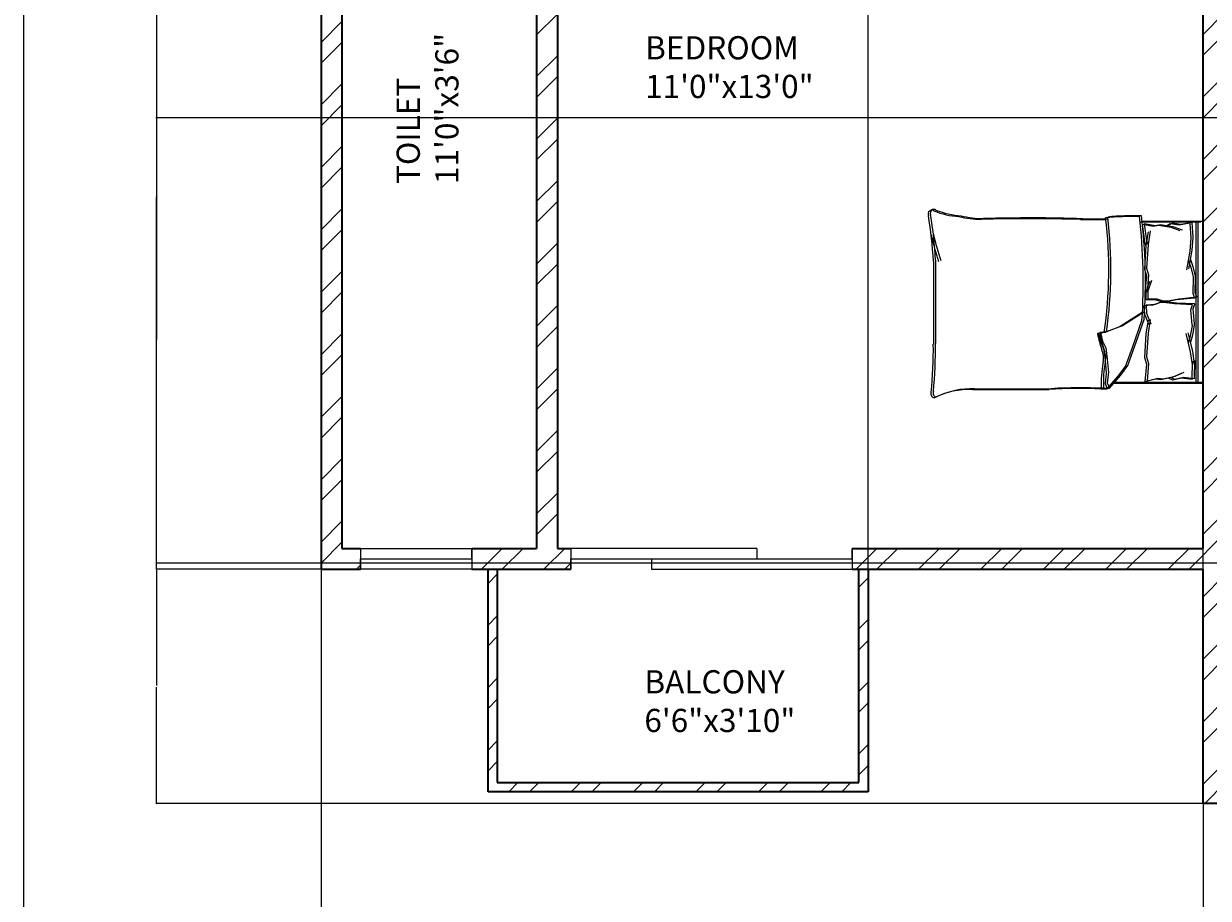
# Model space of a CAD drawing. Units: inches. Extents: x 2064 to 2782, y 1196 to 2299.
# Tile 2 of 11: x 2064 to 2320, y 1620 to 1809. Entities that reach past the tile are written whole.
import ezdxf

# ---------------------------------------------------------------- set-up
doc = ezdxf.new("R2010")
doc.units = ezdxf.units.IN
for name, color, linetype, lineweight in [('A-ANNO-DIMS', 2, 'Continuous', 18), ('A-ANNO-TTLB', 7, 'Continuous', 25), ('A-AREA-IDEN', 7, 'Continuous', 18), ('A-FURN', 8, 'Continuous', 13), ('A-GLAZ', 151, 'Continuous', 18), ('A-WALL', 7, 'Continuous', 35), ('A-WALL-PATT', 9, 'Continuous', 13)]:
    doc.layers.add(name, color=color, linetype=linetype, lineweight=lineweight)
doc.styles.get("Standard").update_dxf_attribs({"font": 'arial.ttf'})
doc.dimstyles.get("Standard").update_dxf_attribs({"dimtxt": 0.18, "dimasz": 0.18, "dimexe": 0.18, "dimexo": 0.0625, "dimgap": 0.09, "dimtad": 0, "dimtih": 1, "dimtoh": 1, "dimdec": 4, "dimzin": 0, "dimdsep": 46, "dimtxsty": 'Standard', "dimcen": 0.09, "dimadec": 0, "dimazin": 0, "dimtfac": 1, "dimtdec": 4, "dimtofl": 0, "dimtmove": 0, "dimatfit": 3, "dimfxl": 1, "dimtolj": 1, "dimtzin": 0, "dimarcsym": 0})

# ---------------------------------------------------------------- blocks, each defined once
blk = doc.blocks.new('BED-DOUBLE')
for p, q in [((2.53, 46.14), (2.53, 59.33)), ((2.53, 46.14), (2.53, 59.33)), ((2.53, 59.33), (37.35, 59.33)), ((2.7, 45.67), (2.7, 58.87)), ((2.7, 45.67), (2.7, 58.87)), ((37.35, 59.33), (37.35, 39.95)), ((37.35, 59.33), (37.35, 39.95)), ((37.52, 59.33), (37.52, 58.87)), ((37.52, 58.87), (37.52, 39.48)), ((37.52, 58.87), (37.52, 39.48)), ((2.53, 58.22), (37.35, 58.22)), ((2.53, 58.22), (37.35, 58.22)), ((2.7, 57.75), (37.52, 57.75)), ((2.7, 57.75), (37.52, 57.75)), ((2.84, 56.9), (5.96, 57.14)), ((2.84, 56.9), (5.96, 57.14)), ((2.84, 56.92), (3.26, 54.6)), ((2.84, 56.92), (3.26, 54.6)), ((3, 56.45), (3.43, 54.14)), ((3, 56.45), (3.43, 54.14)), ((3.01, 56.44), (6.13, 56.68)), ((3.01, 56.44), (6.13, 56.68)), ((5.96, 57.14), (6.04, 57.13)), ((5.96, 57.14), (6.04, 57.13)), ((6.04, 57.13), (8.82, 56.92)), ((6.04, 57.13), (8.82, 56.92)), ((6.13, 56.68), (6.2, 56.66)), ((6.13, 56.68), (6.2, 56.66)), ((6.2, 56.66), (8.99, 56.45)), ((6.2, 56.66), (8.99, 56.45)), ((8.82, 56.92), (12.82, 56.18)), ((8.82, 56.92), (12.82, 56.18)), ((8.99, 56.45), (12.99, 55.72)), ((8.99, 56.45), (12.99, 55.72)), ((10.82, 56.6), (12.3, 57.13)), ((10.82, 56.6), (12.3, 57.13)), ((10.99, 56.14), (12.46, 56.66)), ((10.99, 56.14), (12.46, 56.66)), ((12.3, 57.13), (14.4, 57.66)), ((12.3, 57.13), (14.4, 57.66)), ((12.46, 56.66), (14.57, 57.19)), ((12.46, 56.66), (14.57, 57.19)), ((14.4, 57.66), (14.64, 57.66)), ((14.4, 57.66), (14.64, 57.66)), ((14.57, 57.19), (14.8, 57.19)), ((14.57, 57.19), (14.8, 57.19)), ((14.64, 57.66), (17.88, 57.55)), ((14.64, 57.66), (17.88, 57.55)), ((14.8, 57.19), (18.04, 57.09)), ((14.8, 57.19), (18.04, 57.09)), ((17.88, 57.55), (18.93, 57.97)), ((17.88, 57.55), (18.93, 57.97)), ((18.04, 57.09), (19.1, 57.51)), ((18.04, 57.09), (19.1, 57.51)), ((18.93, 57.97), (19.35, 54.07)), ((18.93, 57.97), (19.35, 54.07)), ((19.1, 57.51), (19.52, 53.61)), ((19.1, 57.51), (19.52, 53.61)), ((20.38, 57.52), (20.2, 53.6)), ((20.38, 57.52), (20.21, 53.6)), ((20.55, 57.05), (20.37, 53.14)), ((20.55, 57.05), (20.37, 53.14)), ((21.46, 57.16), (20.38, 57.52)), ((21.46, 57.16), (20.38, 57.52)), ((21.63, 56.7), (20.55, 57.05)), ((21.63, 56.7), (20.55, 57.05)), ((24.69, 57.47), (21.46, 57.16)), ((24.69, 57.47), (21.46, 57.16)), ((24.85, 57.01), (21.63, 56.7)), ((24.85, 57.01), (21.63, 56.7)), ((24.92, 57.49), (24.69, 57.47)), ((24.92, 57.49), (24.69, 57.47)), ((25.09, 57.02), (24.85, 57.01)), ((25.09, 57.02), (24.85, 57.01)), ((27.05, 57.09), (24.92, 57.49)), ((27.05, 57.09), (24.92, 57.49)), ((27.22, 56.63), (25.09, 57.02)), ((27.22, 56.63), (25.09, 57.02)), ((30.54, 57.1), (26.59, 56.11)), ((30.54, 57.1), (26.59, 56.11)), ((30.7, 56.63), (26.75, 55.65)), ((30.7, 56.63), (26.75, 55.65)), ((28.56, 56.66), (27.05, 57.09)), ((28.56, 56.66), (27.05, 57.09)), ((28.73, 56.19), (27.22, 56.63)), ((28.73, 56.19), (27.22, 56.63)), ((33.3, 57.48), (30.54, 57.1)), ((33.3, 57.48), (30.54, 57.1)), ((33.47, 57.02), (30.7, 56.63)), ((33.47, 57.02), (30.7, 56.63)), ((36.51, 57.47), (32.57, 57.54)), ((32.57, 57.54), (33.3, 57.48)), ((36.51, 57.47), (32.57, 57.54)), ((32.57, 57.54), (33.3, 57.48)), ((36.68, 57.01), (32.74, 57.08)), ((32.74, 57.08), (33.47, 57.02)), ((36.67, 57.01), (32.74, 57.08)), ((32.74, 57.08), (33.47, 57.02)), ((36.51, 57.47), (36.23, 55.13)), ((36.51, 57.47), (36.23, 55.13)), ((36.68, 57.01), (36.4, 54.67)), ((36.67, 57.01), (36.4, 54.67)), ((3.26, 54.6), (2.94, 52.71)), ((3.26, 54.6), (2.94, 52.71)), ((3.43, 54.14), (3.11, 52.24)), ((3.43, 54.14), (3.11, 52.24)), ((3.68, 52.81), (4.42, 54.81)), ((3.68, 52.81), (4.42, 54.81)), ((3.85, 52.34), (4.58, 54.35)), ((3.85, 52.34), (4.58, 54.35)), ((19.35, 54.07), (19.77, 51.76)), ((19.35, 54.07), (19.77, 51.76)), ((35.92, 53.32), (35.06, 55.27)), ((35.92, 53.32), (35.06, 55.27)), ((36.09, 52.85), (35.23, 54.8)), ((36.09, 52.85), (35.23, 54.8)), ((36.23, 55.13), (36.67, 53.26)), ((36.23, 55.13), (36.67, 53.26)), ((36.4, 54.67), (36.83, 52.79)), ((36.4, 54.67), (36.83, 52.79)), ((2.94, 52.71), (3.36, 51.97)), ((2.94, 52.71), (3.36, 51.97)), ((3.11, 52.24), (3.53, 51.5)), ((3.11, 52.24), (3.53, 51.5)), ((3.26, 50.18), (3.68, 52.81)), ((3.26, 50.18), (3.68, 52.81)), ((3.43, 49.71), (3.85, 52.34)), ((3.43, 49.71), (3.85, 52.34)), ((19.52, 53.61), (19.94, 51.29)), ((19.52, 53.61), (19.94, 51.29)), ((19.77, 51.76), (19.77, 50.81)), ((19.77, 51.76), (19.77, 50.81)), ((20.21, 53.6), (19.93, 51.26)), ((20.2, 53.6), (19.93, 51.26)), ((19.93, 51.26), (19.99, 50.32)), ((19.93, 51.26), (19.99, 50.32)), ((19.94, 51.29), (19.94, 50.34)), ((19.94, 51.29), (19.94, 50.34)), ((20.37, 53.14), (20.1, 50.8)), ((20.37, 53.14), (20.1, 50.8)), ((36.51, 50.72), (35.92, 53.32)), ((36.51, 50.72), (35.92, 53.32)), ((36.68, 50.25), (36.09, 52.85)), ((36.67, 50.25), (36.09, 52.85)), ((36.67, 53.26), (36.29, 52.5)), ((36.67, 53.26), (36.29, 52.5)), ((36.83, 52.79), (36.46, 52.03)), ((36.83, 52.79), (36.46, 52.03)), ((3.05, 46.7), (3.47, 49.02)), ((3.05, 46.7), (3.47, 49.02)), ((3.47, 49.02), (3.26, 50.18)), ((3.47, 49.02), (3.26, 50.18)), ((3.64, 48.55), (3.43, 49.71)), ((3.64, 48.55), (3.43, 49.71)), ((19.77, 50.81), (19.35, 49.44)), ((19.77, 50.81), (19.35, 49.44)), ((19.35, 49.44), (19.35, 47.49)), ((19.35, 49.44), (19.35, 47.49)), ((19.94, 50.34), (19.52, 48.97)), ((19.94, 50.34), (19.52, 48.97)), ((19.52, 48.97), (19.52, 47.02)), ((19.52, 48.97), (19.52, 47.02)), ((19.99, 50.32), (20.49, 48.98)), ((19.99, 50.32), (20.49, 48.98)), ((20.1, 50.8), (20.15, 49.85)), ((20.1, 50.8), (20.15, 49.85)), ((20.15, 49.85), (20.66, 48.51)), ((20.15, 49.85), (20.66, 48.51)), ((20.49, 48.98), (20.62, 47.03)), ((20.49, 48.98), (20.62, 47.03)), ((36.37, 49.55), (36.51, 50.72)), ((36.37, 49.55), (36.51, 50.72)), ((36.94, 47.26), (36.37, 49.55)), ((36.94, 47.26), (36.37, 49.55)), ((36.54, 49.08), (36.68, 50.25)), ((36.54, 49.08), (36.67, 50.25)), ((37.1, 46.79), (36.54, 49.08)), ((37.1, 46.79), (36.54, 49.08)), ((6.76, 47.23), (3.05, 46.7)), ((6.76, 47.23), (3.05, 46.7)), ((3.21, 46.24), (3.64, 48.55)), ((3.21, 46.24), (3.64, 48.55)), ((6.93, 46.76), (3.21, 46.24)), ((6.93, 46.76), (3.21, 46.24)), ((4.65, 47.95), (7.59, 47.46)), ((4.65, 47.95), (7.59, 47.46)), ((4.82, 47.48), (7.75, 47)), ((4.82, 47.48), (7.75, 47)), ((7.59, 47.46), (6.76, 47.23)), ((7.59, 47.46), (6.76, 47.23)), ((7.75, 47), (6.93, 46.76)), ((7.75, 47), (6.93, 46.76)), ((7.59, 47.46), (12.69, 47.15)), ((7.59, 47.46), (12.69, 47.15)), ((7.75, 47), (12.86, 46.68)), ((7.75, 47), (12.86, 46.68)), ((12.69, 47.15), (14.12, 47.55)), ((12.69, 47.15), (14.12, 47.55)), ((12.86, 46.68), (14.29, 47.09)), ((12.86, 46.68), (14.29, 47.09)), ((14.12, 47.55), (17.86, 47.26)), ((14.12, 47.55), (17.86, 47.26)), ((14.29, 47.09), (18.03, 46.79)), ((14.29, 47.09), (18.03, 46.79)), ((17.56, 47.49), (15.27, 48.28)), ((17.56, 47.49), (15.27, 48.28)), ((17.73, 47.02), (15.44, 47.82)), ((17.73, 47.02), (15.44, 47.82)), ((19.35, 47.49), (17.56, 47.49)), ((19.35, 47.49), (17.56, 47.49)), ((19.52, 47.02), (17.73, 47.02)), ((19.52, 47.02), (17.73, 47.02)), ((20.62, 47.03), (22.4, 47.14)), ((20.62, 47.03), (22.4, 47.14)), ((20.66, 48.51), (20.78, 46.56)), ((20.66, 48.51), (20.78, 46.56)), ((20.78, 46.56), (22.57, 46.67)), ((20.78, 46.56), (22.57, 46.67)), ((22.05, 46.67), (25.1, 41.94)), ((22.05, 46.67), (25.1, 41.94)), ((22.21, 46.2), (25.26, 41.47)), ((22.21, 46.2), (25.26, 41.47)), ((22.4, 47.14), (24.64, 48.08)), ((22.4, 47.14), (24.64, 48.08)), ((22.57, 46.67), (24.81, 47.61)), ((22.57, 46.67), (24.81, 47.61)), ((29.61, 44.53), (23.54, 46.67)), ((29.61, 44.53), (23.54, 46.67)), ((29.78, 44.07), (23.7, 46.2)), ((29.78, 44.07), (23.7, 46.2)), ((23.72, 47.95), (26.66, 47.46)), ((23.72, 47.95), (26.66, 47.46)), ((23.89, 47.48), (26.83, 47)), ((23.89, 47.48), (26.83, 47)), ((26.66, 47.46), (31.77, 47.15)), ((26.66, 47.46), (31.77, 47.15)), ((26.83, 47), (31.94, 46.68)), ((26.83, 47), (31.94, 46.68)), ((31.77, 47.15), (33.2, 47.55)), ((31.77, 47.15), (33.2, 47.55)), ((31.94, 46.68), (33.36, 47.09)), ((31.94, 46.68), (33.36, 47.09)), ((33.2, 47.55), (36.94, 47.26)), ((33.2, 47.55), (36.94, 47.26)), ((33.36, 47.09), (37.1, 46.79)), ((33.36, 47.09), (37.1, 46.79)), ((33.67, 43.07), (29.61, 44.53)), ((33.67, 43.07), (29.61, 44.53)), ((33.84, 42.6), (29.78, 44.07)), ((33.84, 42.6), (29.78, 44.07)), ((25.1, 41.94), (26.34, 38.67)), ((25.1, 41.94), (26.34, 38.67)), ((25.26, 41.47), (26.51, 38.2)), ((25.26, 41.47), (26.51, 38.2)), ((35.82, 41.49), (33.67, 43.07)), ((35.82, 41.49), (33.67, 43.07)), ((35.98, 41.02), (33.84, 42.6)), ((35.98, 41.02), (33.84, 42.6)), ((38.52, 39.12), (35.82, 41.49)), ((38.52, 39.12), (35.82, 41.49)), ((38.68, 38.65), (35.98, 41.02)), ((38.68, 38.65), (35.98, 41.02)), ((26.34, 38.67), (26.56, 37.2)), ((26.34, 38.67), (26.56, 37.2)), ((29.84, 38.33), (32.32, 38.67)), ((29.84, 38.33), (32.32, 38.67)), ((32.32, 38.67), (35.14, 38.9)), ((32.32, 38.67), (35.14, 38.9)), ((32.49, 38.2), (35.31, 38.43)), ((32.49, 38.2), (35.31, 38.43)), ((35.14, 38.9), (37.4, 38.67)), ((35.14, 38.9), (37.4, 38.67)), ((35.31, 38.43), (37.56, 38.2)), ((35.31, 38.43), (37.56, 38.2)), ((37.4, 38.67), (38.52, 39.12)), ((37.4, 38.67), (38.52, 39.12)), ((37.56, 38.2), (38.68, 38.65)), ((37.56, 38.2), (38.68, 38.65)), ((38.57, 37.85), (38.52, 39.12, 2.82)), ((38.57, 37.85), (38.52, 39.12, 2.82)), ((38.74, 37.38), (38.68, 38.65, 2.82)), ((38.74, 37.38), (38.68, 38.65, 2.82)), ((26.51, 38.2), (26.73, 36.74)), ((26.51, 38.2), (26.73, 36.74)), ((26.56, 37.2), (28.37, 37.65)), ((26.56, 37.2), (28.37, 37.65)), ((26.73, 36.74), (28.54, 37.19)), ((26.73, 36.74), (28.54, 37.19)), ((28.37, 37.65), (29.84, 38.33)), ((28.37, 37.65), (29.84, 38.33)), ((28.54, 37.19), (30, 37.87)), ((28.54, 37.19), (30, 37.87)), ((30, 37.87), (32.49, 38.2)), ((30, 37.87), (32.49, 38.2)), ((10.97, 1.6), (28.91, 1.6)), ((10.97, 1.6), (28.91, 1.6)), ((11.14, 1.14), (29.07, 1.14)), ((11.14, 1.14), (29.07, 1.14))]:
    blk.add_line(p, q)
for centre, radius, start, end in [((62.04, 44.69), 60.69, 178.7218, 185.604), ((62.04, 44.69), 60.69, 178.7218, 185.604), ((15.56, -73.3), 120.19, 86.0865, 96.7821), ((15.56, -73.3), 120.19, 86.0865, 96.7821), ((15.73, -73.76), 120.19, 86.0865, 96.7821), ((15.73, -73.76), 120.19, 86.0865, 96.7821), ((62.21, 44.23), 60.69, 178.7218, 185.604), ((62.21, 44.23), 60.69, 178.7218, 185.604), ((12.94, -54.55), 94, 81.7845, 96.9006), ((12.94, -54.55), 94, 81.7845, 96.9006), ((13.1, -55.01), 94, 81.7845, 96.9006), ((13.1, -55.01), 94, 81.7845, 96.9006), ((-121.89, 36.62), 123.93, 358.4762, 1.0082), ((-121.89, 36.62), 123.93, 358.4762, 1.0082), ((-121.72, 36.16), 123.93, 358.4762, 1.0082), ((-121.72, 36.16), 123.93, 358.4762, 1.0082), ((26.69, 37.16), 0.134, 160.2464, 271.1377), ((26.69, 37.16), 0.134, 160.2464, 271.1377), ((22.7, 58.25), 21.6, 280.6617, 289.8806), ((22.7, 58.25), 21.6, 280.6617, 289.8806), ((26.86, 36.69), 0.134, 160.2464, 271.1377), ((26.86, 36.69), 0.134, 160.2464, 271.1377), ((22.86, 57.79), 21.6, 280.6617, 289.8806), ((22.86, 57.79), 21.6, 280.6617, 289.8806), ((31.87, 33.79), 4.53, 78.6608, 113.7384), ((31.87, 33.79), 4.53, 78.6608, 113.7384), ((32.04, 33.32), 4.53, 78.6608, 113.7384), ((32.04, 33.32), 4.53, 78.6608, 113.7384), ((37.39, 64.18), 26.36, 259.8763, 272.5657), ((37.39, 64.18), 26.36, 259.8763, 272.5657), ((37.56, 63.72), 26.36, 259.8763, 272.5657), ((37.56, 63.72), 26.36, 259.8763, 272.5657), ((132.79, 32.88), 94.35, 176.9791, 183.8365), ((132.79, 32.88), 94.35, 176.9791, 183.8365), ((132.95, 32.41), 94.35, 176.9791, 183.8365), ((132.95, 32.41), 94.35, 176.9791, 183.8365), ((353.21, 22.46), 351.38, 178.2277, 181.7185), ((353.21, 22.46), 351.38, 178.2277, 181.7185), ((353.38, 21.99), 351.38, 178.2277, 181.7185), ((353.38, 21.99), 351.38, 178.2277, 181.7185), ((-3284.8, 9.92), 3323.5, 0.00217, 0.28689), ((-3284.8, 9.92), 3323.5, 0.00217, 0.28689), ((-3284.64, 9.46), 3323.5, 0.00217, 0.28689), ((-3284.64, 9.46), 3323.5, 0.00217, 0.28689), ((-19.6, 12.33), 21.59, 346.0648, 358.9113), ((-19.6, 12.33), 21.59, 346.0648, 358.9113), ((-19.43, 11.87), 21.59, 346.0648, 358.9113), ((-19.43, 11.87), 21.59, 346.0648, 358.9113), ((55.48, 9.31), 16.8, 177.4714, 206.4681), ((55.48, 9.31), 16.8, 177.4714, 206.4681), ((55.65, 8.84), 16.8, 177.4714, 206.4681), ((55.65, 8.84), 16.8, 177.4714, 206.4681), ((-15.78, 8.14), 17.17, 337.9751, 356.652), ((-15.78, 8.14), 17.17, 337.9751, 356.652), ((-15.61, 7.67), 17.17, 337.9751, 356.652), ((-15.61, 7.67), 17.17, 337.9751, 356.652), ((-12.55, 76.61), 77.56, 283.3832, 287.7053), ((-12.55, 76.61), 77.56, 283.3832, 287.7053), ((0.79, 1.26), 0.793, 146.1736, 293.4781), ((0.79, 1.26), 0.793, 146.1736, 293.4781), ((0.96, 0.79), 0.793, 146.1736, 293.4781), ((0.96, 0.79), 0.793, 146.1736, 293.4781), ((15.61, -86.98), 88.71, 92.9958, 99.4091), ((15.61, -86.98), 88.71, 92.9958, 99.4091), ((15.78, -87.45), 88.71, 92.9958, 99.4091), ((15.78, -87.45), 88.71, 92.9958, 99.4091), ((-12.38, 76.14), 77.56, 283.3832, 287.7053), ((-12.38, 76.14), 77.56, 283.3832, 287.7053), ((29.98, -95.32), 96.92, 84.4998, 90.6351), ((29.98, -95.32), 96.92, 84.4998, 90.6351), ((30.15, -95.78), 96.92, 84.4998, 90.6351), ((30.15, -95.78), 96.92, 84.4998, 90.6351), ((39.64, 1.87), 0.803, 242.6588, 356.02), ((39.64, 1.87), 0.803, 242.6588, 356.02), ((39.81, 1.41), 0.803, 242.6588, 356.02), ((39.81, 1.41), 0.803, 242.6588, 356.02)]:
    blk.add_arc(centre, radius, start, end)
blk = doc.blocks.new('*D24')
at = {"layer": 'A-ANNO-DIMS', "color": 0, "lineweight": -2, "transparency": 16777216}
for p, q in [((2128.17, 1691.23), (2128.17, 1539.01)), ((2318.45, 1640.73), (2318.45, 1539.01)), ((2128.35, 1539.19), (2222.93, 1539.19)), ((2318.27, 1539.19), (2223.7, 1539.19))]:
    blk.add_line(p, q, dxfattribs=at)
at = {"layer": 'A-ANNO-DIMS', "color": 0, "transparency": 16777216}
for points in [[(2128.35, 1539.22), (2128.35, 1539.16), (2128.17, 1539.19)], [(2318.27, 1539.22), (2318.27, 1539.16), (2318.45, 1539.19)]]:
    blk.add_solid(points, dxfattribs=at)
at = {"layer": 'Defpoints', "color": 0, "transparency": 16777216}
for p in [(2128.17, 1691.29), (2318.45, 1640.79), (2318.45, 1539.19)]:
    blk.add_point(p, dxfattribs=at)
at = {"layer": 'A-ANNO-DIMS', "color": 0, "transparency": 16777216, "insert": (2223.31, 1539.19), "char_height": 0.18, "attachment_point": 5}
blk.add_mtext('\\A1;190.3', dxfattribs=at)
blk = doc.blocks.new('*D25')
at = {"layer": 'A-ANNO-DIMS', "color": 0, "lineweight": -2, "transparency": 16777216}
for p, q in [((2318.45, 1640.73), (2318.45, 1539.01)), ((2452.17, 1640.73), (2452.17, 1539.01)), ((2318.63, 1539.19), (2384.86, 1539.19)), ((2451.99, 1539.19), (2385.77, 1539.19))]:
    blk.add_line(p, q, dxfattribs=at)
at = {"layer": 'A-ANNO-DIMS', "color": 0, "transparency": 16777216}
for points in [[(2318.63, 1539.22), (2318.63, 1539.16), (2318.45, 1539.19)], [(2451.99, 1539.22), (2451.99, 1539.16), (2452.17, 1539.19)]]:
    blk.add_solid(points, dxfattribs=at)
at = {"layer": 'Defpoints', "color": 0, "transparency": 16777216}
for p in [(2318.45, 1640.79), (2452.17, 1640.79), (2452.17, 1539.19)]:
    blk.add_point(p, dxfattribs=at)
at = {"layer": 'A-ANNO-DIMS', "color": 0, "transparency": 16777216, "insert": (2385.31, 1539.19), "char_height": 0.18, "attachment_point": 5}
blk.add_mtext('\\A1;133.72', dxfattribs=at)
blk = doc.blocks.new('*D26')
at = {"layer": 'A-ANNO-DIMS', "color": 0, "lineweight": -2, "transparency": 16777216}
for p, q in [((2246.18, 1643.35), (2246.18, 2269.97)), ((2246.36, 2269.79), (2281.92, 2269.79)), ((2318.27, 2269.79), (2282.71, 2269.79)), ((2318.45, 1640.85), (2318.45, 2269.97))]:
    blk.add_line(p, q, dxfattribs=at)
at = {"layer": 'A-ANNO-DIMS', "color": 0, "transparency": 16777216}
for points in [[(2246.36, 2269.82), (2246.36, 2269.76), (2246.18, 2269.79)], [(2318.27, 2269.82), (2318.27, 2269.76), (2318.45, 2269.79)]]:
    blk.add_solid(points, dxfattribs=at)
at = {"layer": 'Defpoints', "color": 0, "transparency": 16777216}
for p in [(2318.45, 2269.79), (2246.18, 1643.29), (2318.45, 1640.79)]:
    blk.add_point(p, dxfattribs=at)
at = {"layer": 'A-ANNO-DIMS', "color": 0, "transparency": 16777216, "insert": (2282.32, 2269.79), "char_height": 0.18, "attachment_point": 5}
blk.add_mtext('\\A1;72.27', dxfattribs=at)
blk = doc.blocks.new('*D28')
at = {"layer": 'A-ANNO-DIMS', "color": 0, "lineweight": -2, "transparency": 16777216}
for p, q in [((2128.11, 1691.29), (2092.49, 1691.29)), ((2092.67, 1691.11), (2092.67, 1666.22)), ((2092.67, 1640.97), (2092.67, 1665.86)), ((2318.39, 1640.79), (2092.49, 1640.79))]:
    blk.add_line(p, q, dxfattribs=at)
at = {"layer": 'A-ANNO-DIMS', "color": 0, "transparency": 16777216}
for points in [[(2092.64, 1691.11), (2092.7, 1691.11), (2092.67, 1691.29)], [(2092.64, 1640.97), (2092.7, 1640.97), (2092.67, 1640.79)]]:
    blk.add_solid(points, dxfattribs=at)
at = {"layer": 'Defpoints', "color": 0, "transparency": 16777216}
for p in [(2092.67, 1691.29), (2128.17, 1691.29), (2318.45, 1640.79)]:
    blk.add_point(p, dxfattribs=at)
at = {"layer": 'A-ANNO-DIMS', "color": 0, "transparency": 16777216, "insert": (2092.67, 1666.04), "char_height": 0.18, "attachment_point": 5}
blk.add_mtext('\\A1;50.5', dxfattribs=at)
blk = doc.blocks.new('*D29')
at = {"layer": 'A-ANNO-DIMS', "color": 0, "lineweight": -2, "transparency": 16777216}
for p, q in [((2132.61, 1851.79), (2092.49, 1851.79)), ((2092.67, 1851.61), (2092.67, 1771.72)), ((2092.67, 1691.47), (2092.67, 1771.36)), ((2128.11, 1691.29), (2092.49, 1691.29))]:
    blk.add_line(p, q, dxfattribs=at)
at = {"layer": 'A-ANNO-DIMS', "color": 0, "transparency": 16777216}
for points in [[(2092.64, 1851.61), (2092.7, 1851.61), (2092.67, 1851.79)], [(2092.64, 1691.47), (2092.7, 1691.47), (2092.67, 1691.29)]]:
    blk.add_solid(points, dxfattribs=at)
at = {"layer": 'Defpoints', "color": 0, "transparency": 16777216}
for p in [(2092.67, 1851.79), (2132.67, 1851.79), (2128.17, 1691.29)]:
    blk.add_point(p, dxfattribs=at)
at = {"layer": 'A-ANNO-DIMS', "color": 0, "transparency": 16777216, "insert": (2092.67, 1771.54), "char_height": 0.18, "attachment_point": 5}
blk.add_mtext('\\A1;160.5', dxfattribs=at)
blk = doc.blocks.new('*D37')
at = {"layer": 'A-ANNO-DIMS', "color": 0, "lineweight": -2, "transparency": 16777216}
for p, q in [((2447.61, 1788.61), (2092.49, 1788.61)), ((2092.67, 1788.43), (2092.67, 1740.79)), ((2092.67, 1692.79), (2092.67, 1740.43)), ((2447.61, 1692.61), (2092.49, 1692.61))]:
    blk.add_line(p, q, dxfattribs=at)
at = {"layer": 'A-ANNO-DIMS', "color": 0, "transparency": 16777216}
for points in [[(2092.64, 1788.43), (2092.7, 1788.43), (2092.67, 1788.61)], [(2092.64, 1692.79), (2092.7, 1692.79), (2092.67, 1692.61)]]:
    blk.add_solid(points, dxfattribs=at)
at = {"layer": 'Defpoints', "color": 0, "transparency": 16777216}
for p in [(2092.67, 1788.61), (2447.67, 1788.61), (2447.67, 1692.61)]:
    blk.add_point(p, dxfattribs=at)
at = {"layer": 'A-ANNO-DIMS', "color": 0, "transparency": 16777216, "insert": (2092.67, 1740.61), "char_height": 0.18, "attachment_point": 5}
blk.add_mtext('\\A1;96', dxfattribs=at)

msp = doc.modelspace()

# ---------------------------------------------------------------- hatches: boundary and pattern name
at = {"layer": 'A-WALL-PATT'}
h = msp.add_hatch(dxfattribs=at)
h.set_pattern_fill('ANSI32', color=256)
h.paths.add_polyline_path([(2489.7688, 2189.2917), (2574.5454, 2189.2917), (2574.5454, 2191.5417), (2574.5454, 2193.7917), (2570.6691, 2193.7917), (2570.6691, 2197.3052), (2568.4191, 2197.3052), (2566.1691, 2197.3052), (2566.1691, 2193.7917), (2494.1691, 2193.7917), (2494.1691, 2229.7917), (2523.2441, 2229.7917), (2523.2441, 2234.2917), (2471.2886, 2234.2917), (2471.2886, 2229.7917), (2489.6691, 2229.7917), (2489.6691, 2193.7917), (2417.6691, 2193.7917), (2417.6691, 2197.0632), (2415.4191, 2197.0632), (2413.1691, 2197.0632), (2413.1691, 2193.7917), (2406.8865, 2193.7917), (2406.8865, 2189.2917), (2485.2688, 2189.2917), (2485.2688, 2063.2917), (2369.1629, 2063.2917), (2369.1629, 2058.7917), (2386.1222, 2058.7917), (2386.1222, 1856.2917), (2382.1576, 1856.2917), (2382.1576, 1851.7917), (2394.9764, 1851.7917), (2394.9764, 1854.0417), (2394.9764, 1856.2917), (2390.6222, 1856.2917), (2390.6222, 2058.7917), (2485.2688, 2058.7917), (2493.762, 2058.7917), (2493.762, 2061.0417), (2493.762, 2063.2917), (2489.7688, 2063.2917)])
h.paths.add_polyline_path([(2447.2886, 2234.2917), (2413.1691, 2234.2917), (2413.1691, 2217.3799), (2417.6691, 2217.3799), (2417.6691, 2229.7917), (2447.2886, 2229.7917)], flags=17)
h.paths.add_polyline_path([(2570.6691, 2234.2917), (2547.2441, 2234.2917), (2547.2441, 2229.7917), (2566.1691, 2229.7917), (2566.1691, 2216.5615), (2570.6691, 2216.5615)], flags=17)
h.paths.add_polyline_path([(2653.1691, 2189.2917), (2653.1691, 2193.7917), (2640.8843, 2193.7917), (2640.8843, 2189.2917), (2648.6691, 2189.2917), (2648.6691, 2162.7138), (2653.1691, 2162.7138)])
h.paths.add_polyline_path([(2653.1691, 2102.7138), (2648.6691, 2102.7138), (2648.6691, 2063.2917), (2526.7281, 2063.2917), (2526.7281, 2058.7917), (2541.1691, 2058.7917), (2541.1691, 1993.2917), (2545.6691, 1993.2917), (2545.6691, 1997.7917), (2545.6691, 2058.7917), (2648.6691, 2058.7917), (2648.6691, 2050.1099), (2653.1691, 2050.1099)])
h.paths.add_polyline_path([(2600.6691, 1856.2917), (2493.4607, 1856.2917), (2493.4607, 1851.7917), (2596.1691, 1851.7917), (2596.1691, 1695.7917), (2594.0816, 1695.7917), (2594.0816, 1691.2917), (2614.7905, 1691.2917), (2614.7905, 1645.2917), (2536.7905, 1645.2917), (2536.7905, 1691.2917), (2539.332, 1691.2917), (2539.332, 1693.5417), (2539.332, 1695.7917), (2452.1691, 1695.7917), (2452.1691, 1851.7917), (2456.0775, 1851.7917), (2456.0775, 1856.2917), (2427.1536, 1856.2917), (2427.1536, 1851.7917), (2447.6691, 1851.7917), (2447.6691, 1695.7917), (2447.6691, 1645.2917), (2405.1469, 1645.2917), (2405.1469, 1640.7917), (2452.1691, 1640.7917), (2452.1691, 1645.2917), (2452.1691, 1691.2917), (2534.7905, 1691.2917), (2534.7905, 1645.2917), (2534.7905, 1643.2917), (2614.7905, 1643.2917), (2616.7905, 1643.2917), (2616.7905, 1691.2917), (2622.4029, 1691.2917), (2622.4029, 1693.7143), (2622.4029, 1695.7917), (2600.6691, 1695.7917), (2600.6691, 1779.7917), (2648.6691, 1779.7917), (2648.6691, 1695.7917), (2646.4029, 1695.7917), (2646.4029, 1691.2917), (2653.1691, 1691.2917), (2653.1691, 1906.3508), (2648.6691, 1906.3508), (2648.6691, 1856.2917), (2648.6691, 1784.2917), (2600.6691, 1784.2917)])
h.paths.add_polyline_path([(2322.9532, 1819.5181), (2320.7032, 1819.5181), (2318.4532, 1819.5181), (2318.4532, 1695.7917), (2242.7664, 1695.7917), (2242.7664, 1691.2917), (2318.4532, 1691.2917), (2318.4532, 1640.7917), (2322.9532, 1640.7917), (2345.1469, 1640.7917), (2345.1469, 1643.0417), (2345.1469, 1645.2917), (2322.9532, 1645.2917), (2322.9532, 1691.2917), (2322.9532, 1695.7917)])
h.paths.add_polyline_path([(2166.1825, 1691.2917), (2164.1825, 1691.2917), (2164.1825, 1643.2917), (2166.1825, 1643.2917), (2246.1825, 1643.2917), (2246.1825, 1645.2917), (2246.1825, 1691.2917), (2244.1825, 1691.2917), (2244.1825, 1645.2917), (2166.1825, 1645.2917)])
h.paths.add_polyline_path([(2309.404, 1932.7917), (2204.1691, 1932.7917), (2204.1691, 1960.0962), (2199.6691, 1960.0962), (2199.6691, 1932.7917), (2132.6691, 1932.7917), (2132.6691, 1951.0737), (2128.1691, 1951.0737), (2128.1691, 1910.0412), (2132.6691, 1910.0412), (2132.6691, 1928.2917), (2304.904, 1928.2917), (2304.904, 1856.2917), (2304.904, 1851.7917), (2318.4532, 1851.7917), (2318.4532, 1848.8308), (2322.9532, 1848.8308), (2322.9532, 1851.7917), (2347.7631, 1851.7917), (2347.7631, 1856.2917), (2309.404, 1856.2917)])
h.paths.add_polyline_path([(2132.6691, 2044.9092), (2130.4191, 2044.9092), (2128.1691, 2044.9092), (2128.1691, 1987.0737), (2132.6691, 1987.0737), (2132.6691, 2004.7917), (2199.6691, 2004.7917), (2204.1691, 2004.7917), (2204.1691, 2009.2917), (2132.6691, 2009.2917)])
h.paths.add_polyline_path([(2186.6691, 2195.9329), (2184.4191, 2195.9329), (2184.4191, 2195.8929), (2182.1691, 2195.9329), (2182.1691, 2193.7917), (2128.1691, 2193.7917), (2128.1691, 2181.4967), (2132.6691, 2181.4967), (2132.6691, 2182.7769), (2132.6691, 2189.2917), (2182.1691, 2189.2917), (2182.1691, 2135.2917), (2179.804, 2135.2917), (2179.804, 2130.7917), (2190.215, 2130.7917), (2190.215, 2133.0417), (2190.215, 2135.2917), (2186.6691, 2135.2917)])
h.paths.add_polyline_path([(2340.0628, 2189.2917), (2340.0628, 2191.5417), (2340.0628, 2193.7917), (2335.1691, 2193.7917), (2335.1691, 2234.2917), (2280.6746, 2234.2917), (2280.6746, 2229.7917), (2330.6691, 2229.7917), (2330.6691, 2193.7917), (2330.6691, 2135.2917), (2218.6309, 2135.2917), (2218.6309, 2130.7917), (2330.7688, 2130.7917), (2330.7688, 2008.4023), (2335.2688, 2008.4023), (2335.2688, 2058.7917), (2338.9208, 2058.7917), (2338.9208, 2061.0417), (2338.9208, 2063.2917), (2335.2688, 2063.2917), (2335.2688, 2189.2917)])
h.paths.add_polyline_path([(2220.6746, 2234.2917), (2182.1691, 2234.2917), (2182.1691, 2227.4187), (2186.6691, 2227.4187), (2186.6691, 2229.7917), (2220.6746, 2229.7917), (2220.6746, 2232.0417)])
h.paths.add_polyline_path([(2158.8146, 2135.2917), (2132.6691, 2135.2917), (2132.6691, 2157.4967), (2128.1691, 2157.4967), (2128.1691, 2104.9092), (2132.6691, 2104.9092), (2132.6691, 2130.7917), (2158.8146, 2130.7917), (2158.8146, 2133.0417)])
h.paths.add_polyline_path([(2396.0464, 2062.2045), (2434.8868, 2062.2045), (2434.8868, 2080.8619), (2396.0464, 2080.8619)], flags=24)
h.paths.add_polyline_path([(2196.1396, 1653.3449), (2232.023, 1653.3449), (2232.023, 1672.0022), (2196.1396, 1672.0022)], flags=25)
h = msp.add_hatch(dxfattribs=at)
h.set_pattern_fill('ANSI32', color=256)
h.paths.add_polyline_path([(2225.5529, 1856.2917), (2132.6691, 1856.2917), (2132.6691, 1874.0412), (2130.4191, 1874.0412), (2128.1691, 1874.0412), (2128.1691, 1691.2917), (2136.6659, 1691.2917), (2136.6659, 1693.5417), (2136.6659, 1695.7917), (2132.6691, 1695.7917), (2132.6691, 1851.7917), (2174.6691, 1851.7917), (2174.6691, 1847.1454), (2179.1691, 1847.1454), (2179.1691, 1851.7917), (2225.5529, 1851.7917)])
h.paths.add_polyline_path([(2179.1691, 1825.2823), (2176.9191, 1825.2823), (2174.6691, 1825.2823), (2174.6691, 1695.7917), (2160.6659, 1695.7917), (2160.6659, 1691.2917), (2182.0177, 1691.2917), (2182.0177, 1693.5417), (2182.0177, 1695.7917), (2179.1691, 1695.7917)], flags=17)

# ---------------------------------------------------------------- linework, layer by layer
at = {"layer": 'A-ANNO-TTLB'}
msp.add_lwpolyline([(2063.9994, 2298.574), (2782.0941, 2298.574), (2782.0941, 1490.6238), (2063.9994, 1490.6238)], close=True, dxfattribs=at)
at = {"layer": 'A-GLAZ'}
for p, q in [((2136.6659, 1695.7917), (2136.6659, 1691.2917)), ((2136.6659, 1695.7917), (2160.6659, 1695.7917)), ((2160.6659, 1693.5417), (2160.6659, 1695.7917)), ((2160.6659, 1695.7917), (2160.6659, 1691.2917)), ((2182.0177, 1695.7917), (2182.0177, 1691.2917)), ((2183.1847, 1695.7917), (2182.0177, 1695.7917)), ((2222.1613, 1695.7917), (2183.1847, 1695.7917)), ((2222.1613, 1695.7917), (2222.1613, 1693.5417)), ((2242.7664, 1693.5417), (2242.7664, 1695.7917)), ((2242.7664, 1695.7917), (2242.7664, 1691.2917)), ((2136.6659, 1691.2917), (2136.6659, 1693.5417)), ((2136.6659, 1693.5417), (2160.6659, 1693.5417)), ((2182.0177, 1691.2917), (2182.0177, 1693.5417)), ((2182.0177, 1693.5417), (2242.7664, 1693.5417)), ((2199.4738, 1693.5417), (2199.4738, 1691.2917)), ((2160.6659, 1691.2917), (2136.6659, 1691.2917)), ((2199.4738, 1691.2917), (2242.7664, 1691.2917))]:
    msp.add_line(p, q, dxfattribs=at)
at = {"layer": 'A-WALL'}
for p, q in [((2128.1691, 1874.0412), (2128.1691, 1691.2917)), ((2132.6691, 1851.7917), (2132.6691, 1695.7917)), ((2174.6691, 1826.7576), (2174.6691, 1695.7917)), ((2179.1691, 1825.2823), (2179.1691, 1695.7917)), ((2318.4532, 1695.7917), (2318.4532, 1820.8188)), ((2132.6691, 1695.7917), (2136.6659, 1695.7917)), ((2160.6659, 1695.7917), (2174.6691, 1695.7917)), ((2179.1691, 1695.7917), (2182.0177, 1695.7917)), ((2242.7664, 1695.7917), (2318.4532, 1695.7917)), ((2128.1691, 1691.2917), (2136.6659, 1691.2917)), ((2160.6659, 1691.2917), (2182.0177, 1691.2917)), ((2164.1825, 1643.2917), (2164.1825, 1691.2917)), ((2166.1825, 1691.2917), (2166.1825, 1645.2917)), ((2242.7664, 1691.2917), (2318.4532, 1691.2917)), ((2244.1825, 1645.2917), (2244.1825, 1691.2917)), ((2244.1825, 1691.2917), (2246.1825, 1691.2917)), ((2246.1825, 1691.2917), (2246.1825, 1645.2917)), ((2318.4532, 1640.7917), (2318.4532, 1691.2917)), ((2166.1825, 1645.2917), (2244.1825, 1645.2917)), ((2246.1825, 1645.2917), (2246.1825, 1643.2917)), ((2166.1825, 1643.2917), (2164.1825, 1643.2917)), ((2246.1825, 1643.2917), (2166.1825, 1643.2917)), ((2322.9532, 1640.7917), (2318.4532, 1640.7917))]:
    msp.add_line(p, q, dxfattribs=at)

# ---------------------------------------------------------------- block references
at = {"layer": 'A-FURN', "rotation": 269.9999998331858}
msp.add_blockref('BED-DOUBLE', (2259.1185, 1768.8664), dxfattribs=at)

# ---------------------------------------------------------------- texts
at = {"layer": 'A-AREA-IDEN', "insert": (2144.4676, 1774.3389), "char_height": 5, "attachment_point": 1, "rotation": 90}
msp.add_mtext_dynamic_manual_height_columns('TOILET\\P11\'0"x3\'6"', width=189.659492, gutter_width=12.5, heights=[0], dxfattribs=at)
at = {"layer": 'A-AREA-IDEN', "char_height": 5, "attachment_point": 1}
for s, width, insert in [('BEDROOM\\P11\'0"x13\'0"', 208.084738, (2198.0595, 1806.2155)), ('BALCONY\\P6\'6"x3\'10"', 113.979526, (2197.9012, 1669.5176))]:
    msp.add_mtext_dynamic_manual_height_columns(s, width=width, gutter_width=12.5, heights=[0], dxfattribs=dict(at, insert=insert))

# ---------------------------------------------------------------- dimensions: what is measured, and where the dimension line sits
at = {"layer": 'A-ANNO-DIMS'}
for base, p1, p2, override, picture, middle in [((2318.4532, 2269.7917), (2246.1825, 1643.2917), (2318.4532, 1640.7917), {"dimdec": 2, "dimlfac": 1, "dimrnd": 0, "dimzin": 0, "dimdsep": 46, "dimlunit": 2}, '*D26', (2282.3178, 2269.7917)), ((2318.4532, 1539.1896), (2128.1691, 1691.2917), (2318.4532, 1640.7917), {"dimdec": 1, "dimlfac": 1, "dimrnd": 0, "dimzin": 0, "dimdsep": 46, "dimlunit": 2}, '*D24', (2223.3112, 1539.1896)), ((2452.1691, 1539.1896), (2318.4532, 1640.7917), (2452.1691, 1640.7917), {"dimdec": 2, "dimlfac": 1, "dimrnd": 0, "dimzin": 0, "dimdsep": 46, "dimlunit": 2}, '*D25', (2385.3112, 1539.1896))]:
    dim = msp.add_linear_dim(base=base, p1=p1, p2=p2, dimstyle='Standard', override=override, dxfattribs=at)
    dim.commit()
    dim.dimension.update_dxf_attribs({"geometry": picture, "text_midpoint": middle})
for base, p1, p2, override, picture, middle in [((2092.6691, 1851.7917), (2128.1691, 1691.2917), (2132.6691, 1851.7917), {"dimdec": 1, "dimlfac": 1, "dimrnd": 0, "dimzin": 0, "dimdsep": 46, "dimlunit": 2}, '*D29', (2092.6691, 1771.5417)), ((2092.6691, 1788.6099), (2447.6691, 1692.6099), (2447.6691, 1788.6099), {"dimdec": 0, "dimlfac": 1, "dimrnd": 0, "dimzin": 0, "dimdsep": 46, "dimlunit": 2}, '*D37', (2092.6691, 1740.6099)), ((2092.6691, 1691.2917), (2318.4532, 1640.7917), (2128.1691, 1691.2917), {"dimdec": 1, "dimlfac": 1, "dimrnd": 0, "dimzin": 0, "dimdsep": 46, "dimlunit": 2}, '*D28', (2092.6691, 1666.0417))]:
    dim = msp.add_linear_dim(base=base, p1=p1, p2=p2, angle=90, dimstyle='Standard', override=override, dxfattribs=at)
    dim.commit()
    dim.dimension.update_dxf_attribs({"geometry": picture, "text_midpoint": middle})

doc.saveas('drawing.dxf')
